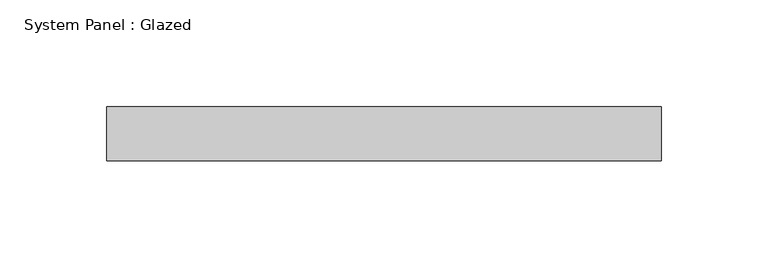
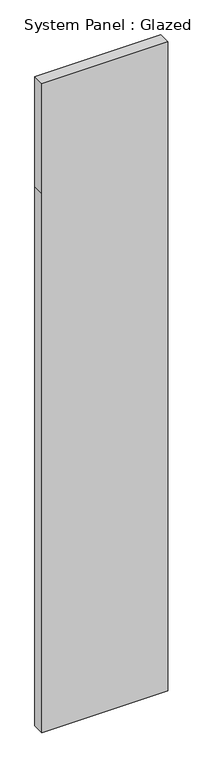
"""IFC4 building model written with IfcOpenShell, lengths in millimetres: plate geometry, System Panel : Glazed."""

from ifc_helpers import new_model, si_unit, frame, origin, place, context, project, spatial, polyline, outline, extrude, source, transform, mapped, element, save


def system_panel_glazed_28683af0(model_context):
    return source(origin(), model_context, "Body", "SweptSolid", [
        extrude(outline(polyline([(0.0, -130.175), (0.0, 130.175), (1181.1, 130.175), (1422.4, 130.175), (1422.4, -130.175), (1181.1, -130.175), (0.0, -130.175)])), frame((0.0, 19.05, 0.0), z_axis=(0.0, 1.0, 0.0), x_axis=(0.0, 0.0, 1.0)), (0.0, 0.0, 1.0), 25.4),
    ])


if __name__ == "__main__":
    model = new_model("IFC4")
    model_context = context("Model", 3, world=origin())
    ifc_project = project(units=[si_unit("LENGTHUNIT", "METRE", prefix="MILLI")], contexts=[model_context])
    site = spatial("IfcSite", under=ifc_project)
    building = spatial("IfcBuilding", under=site)
    placement = place(None, origin())
    system_panel_glazed_shape = system_panel_glazed_28683af0(model_context)
    element("IfcPlate", 1, ObjectType="System Panel : Glazed", at=placement, inside=building, context=model_context, shape_type="MappedRepresentation", body=[
        mapped(system_panel_glazed_shape, transform((0.0, 0.0, 0.0), x_axis=(1.0, 0.0, 0.0), y_axis=(0.0, 1.0, 0.0), z_axis=(0.0, 0.0, 1.0))),
    ])
    save(model, "model.ifc")

# Revit data of these elements
# Type "System Panel : Glazed"
#   Construction Type Id = "GSP4R"
#   Analytic Construction = "1/8 in Pilkington single glazing"
#   Visual Light Transmittance = 0.9
#   Solar Heat Gain Coefficient = 0.86
#   Heat Transfer Coefficient (U) = 1.18115 BTU/(h·ft²·°F)
#   Define Thermal Properties by = 1
# Element 1 (IfcPlate, "System Panel : Glazed")
#   Materials on its faces: "Glass"
# Materials
#   "Glass": class "Glass", colour RGB 0 128 192, transparency 0.75, Description = "Soda Lime Glass", Cost = 0
